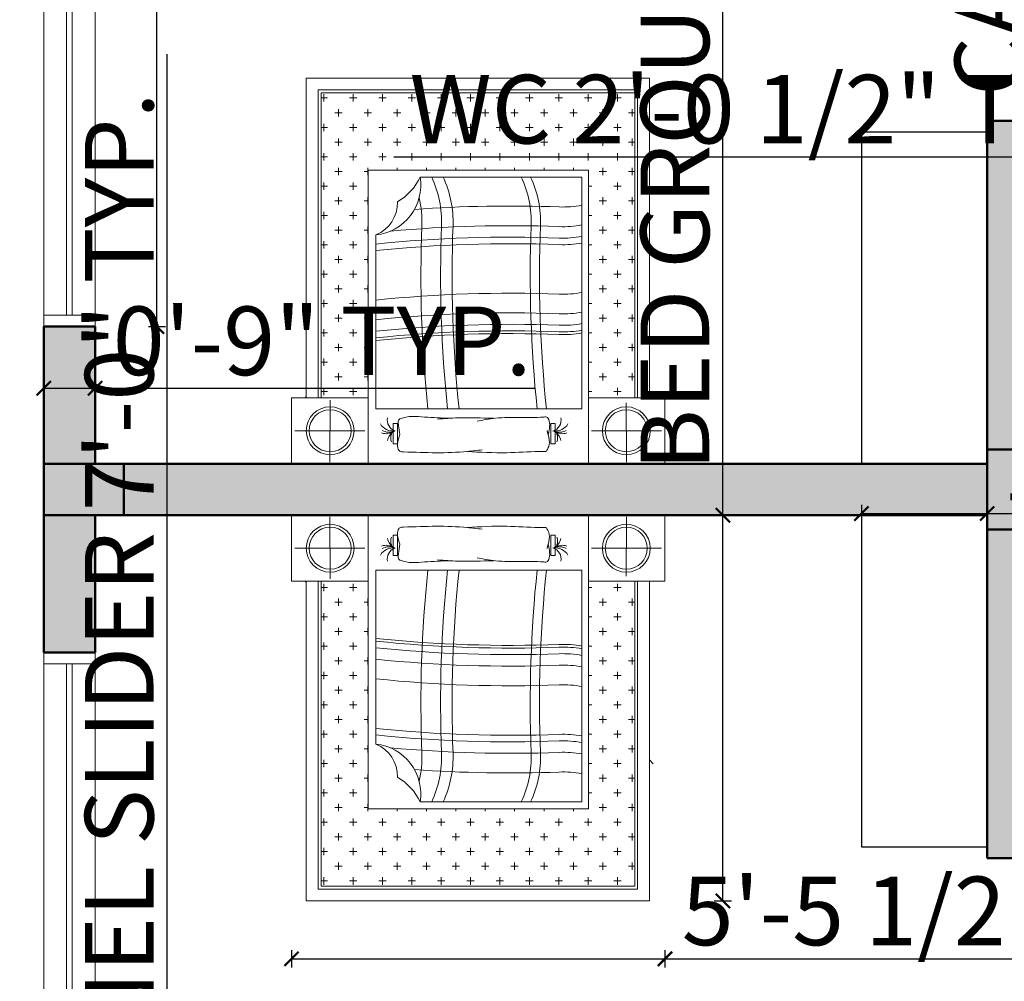
# Model space of a CAD drawing. Units: inches. Extents: x 375 to 1122, y 27 to 1069.
# Tile 71 of 155: x 494 to 667, y 499 to 667. Entities that reach past the tile are written whole.
import ezdxf

# ---------------------------------------------------------------- set-up
doc = ezdxf.new("R2010")
doc.units = ezdxf.units.IN
for name, color, linetype, lineweight in [('A-ANNO-DIMS', 2, 'Continuous', 18), ('A-COLS-PATT', 10, 'Continuous', 13), ('A-FLOR-MILL', 55, 'Continuous', 25), ('A-WALL-PATT', 252, 'Continuous', 13), ('Columns', 10, 'Continuous', 50), ('Doors', 150, 'Continuous', 25), ('Furniture', 30, 'Continuous', 18), ('Walls', 250, 'Continuous', 50), ('Windows', 122, 'Continuous', 18)]:
    doc.layers.add(name, color=color, linetype=linetype, lineweight=lineweight)
doc.styles.get("Standard").update_dxf_attribs({"font": 'arial.ttf'})
doc.dimstyles.new('ISO-25', dxfattribs={"dimtxt": 12, "dimasz": 2.5, "dimexe": 1.5, "dimexo": 1.5, "dimtad": 1, "dimdec": 1, "dimlunit": 3, "dimtxsty": 'Standard', "dimblk": 'ARCHTICK', "dimcen": 2.5, "dimadec": 0, "dimazin": 0, "dimtfac": 1, "dimtdec": 1, "dimtmove": 0, "dimatfit": 3, "dimfxl": 1.5, "dimfxlon": 1, "dimarcsym": 0})

# ---------------------------------------------------------------- blocks, each defined once
blk = doc.blocks.new('*U12')
for p, q in [((0, 0), (0, -4)), ((24, 0), (24, -4))]:
    blk.add_line(p, q)
blk.add_lwpolyline([(0, 0), (0, 24), (1.75, 24), (1.75, 0)], close=True)
blk.add_arc((0, 0), 24, 0, 90)
blk = doc.blocks.new('*U11')
for p, q in [((-24, 0), (-24, -4)), ((0, 0), (0, -4))]:
    blk.add_line(p, q)
blk.add_lwpolyline([(0, 0), (0, 24), (-1.75, 24), (-1.75, 0)], close=True)
blk.add_arc((0, 0), 24, 90, 180)
blk = doc.blocks.new('A$C52B64FF5')
for p, q in [((0.5216, 2.6276), (0, 2.6276)), ((0, 2.6276), (0, 2.1776)), ((0.2616, 2.4026), (0.2616, 2.6161)), ((0.5216, 2.1776), (0.5216, 2.6276)), ((2.0216, 2.6276), (0.5216, 2.6276)), ((0.5216, 2.6276), (0.5216, 0.6276)), ((2.5432, 2.6276), (2.0216, 2.6276)), ((2.0216, 0.6276), (2.0216, 2.6276)), ((2.0216, 2.6276), (2.0216, 2.1776)), ((2.2816, 2.4026), (2.2816, 2.6161)), ((2.5432, 2.1776), (2.5432, 2.6276)), ((0.721, 2.4927), (0.6917, 2.4927)), ((0.6917, 2.4927), (0.6917, 2.3531)), ((0.721, 2.3531), (0.721, 2.4927)), ((1.767, 2.3531), (1.767, 2.4927)), ((1.767, 2.4927), (1.7964, 2.4927)), ((1.7964, 2.4927), (1.7964, 2.3531)), ((0.2632, 2.4026), (0.0233, 2.4026)), ((0.0233, 2.4026), (0.4999, 2.4026)), ((0.2632, 2.1952), (0.2632, 2.4026)), ((0.6917, 2.3531), (0.721, 2.3531)), ((1.7964, 2.3531), (1.767, 2.3531)), ((2.5199, 2.4026), (2.0434, 2.4026)), ((2.2801, 2.2128), (2.2801, 2.4026)), ((2.2801, 2.4026), (2.5199, 2.4026)), ((0.5751, 1.0685), (0.5751, 2.2541)), ((0.5751, 2.2541), (1.9782, 2.2541)), ((1.9782, 2.2541), (1.9782, 0.6749)), ((0, 2.1776), (0.5216, 2.1776)), ((0.093, 2.1776), (0.1008, 2.1698)), ((0.1008, 0), (0.1008, 2.1776)), ((0.1808, 0.08), (0.1808, 2.1776)), ((0.2008, 0.1), (0.2008, 2.1776)), ((0.2197, 2.111), (0.2197, 2.161)), ((0.4197, 2.111), (0.4197, 2.161)), ((2.5432, 2.1776), (2.0216, 2.1776)), ((2.0216, 2.1776), (2.5432, 2.1776)), ((2.2197, 2.111), (2.2197, 2.161)), ((2.3374, 2.1776), (2.3374, 0.1)), ((2.3574, 2.1776), (2.3574, 0.08)), ((2.4374, 2.1776), (2.4374, 0)), ((0.2008, 2.136), (0.2447, 2.136)), ((0.3947, 2.136), (0.4447, 2.136)), ((2.0216, 2.136), (2.0447, 2.136)), ((2.1947, 2.136), (2.2447, 2.136)), ((0.2947, 2.036), (0.3447, 2.036)), ((0.3197, 2.011), (0.3197, 2.061)), ((0.4947, 2.036), (0.5216, 2.036)), ((0.5197, 2.011), (0.5197, 2.061)), ((2.0947, 2.036), (2.1447, 2.036)), ((2.1197, 2.011), (2.1197, 2.061)), ((2.2947, 2.036), (2.3374, 2.036)), ((2.3197, 2.011), (2.3197, 2.061)), ((0.2197, 1.911), (0.2197, 1.961)), ((0.4197, 1.911), (0.4197, 1.961)), ((2.2197, 1.911), (2.2197, 1.961)), ((0.2008, 1.936), (0.2447, 1.936)), ((0.3947, 1.936), (0.4447, 1.936)), ((2.0216, 1.936), (2.0447, 1.936)), ((2.1947, 1.936), (2.2447, 1.936)), ((0.2947, 1.836), (0.3447, 1.836)), ((0.3197, 1.811), (0.3197, 1.861)), ((0.4947, 1.836), (0.5216, 1.836)), ((0.5197, 1.811), (0.5197, 1.861)), ((2.0947, 1.836), (2.1447, 1.836)), ((2.1197, 1.811), (2.1197, 1.861)), ((2.2947, 1.836), (2.3374, 1.836)), ((2.3197, 1.811), (2.3197, 1.861)), ((0.2197, 1.711), (0.2197, 1.761)), ((0.4197, 1.711), (0.4197, 1.761)), ((2.2197, 1.711), (2.2197, 1.761)), ((0.2008, 1.736), (0.2447, 1.736)), ((0.3947, 1.736), (0.4447, 1.736)), ((2.0216, 1.736), (2.0447, 1.736)), ((2.1947, 1.736), (2.2447, 1.736)), ((0.2947, 1.636), (0.3447, 1.636)), ((0.3197, 1.611), (0.3197, 1.661)), ((0.4947, 1.636), (0.5216, 1.636)), ((0.5197, 1.611), (0.5197, 1.661)), ((2.0947, 1.636), (2.1447, 1.636)), ((2.1197, 1.611), (2.1197, 1.661)), ((2.2947, 1.636), (2.3374, 1.636)), ((2.3197, 1.611), (2.3197, 1.661)), ((0.2197, 1.511), (0.2197, 1.561)), ((0.4197, 1.511), (0.4197, 1.561)), ((2.2197, 1.511), (2.2197, 1.561)), ((0.2008, 1.536), (0.2447, 1.536)), ((0.3947, 1.536), (0.4447, 1.536)), ((2.0216, 1.536), (2.0447, 1.536)), ((2.1947, 1.536), (2.2447, 1.536)), ((0.2947, 1.436), (0.3447, 1.436)), ((0.3197, 1.411), (0.3197, 1.461)), ((0.4947, 1.436), (0.5216, 1.436)), ((0.5197, 1.411), (0.5197, 1.461)), ((2.0947, 1.436), (2.1447, 1.436)), ((2.1197, 1.411), (2.1197, 1.461)), ((2.2947, 1.436), (2.3374, 1.436)), ((2.3197, 1.411), (2.3197, 1.461)), ((0.2197, 1.311), (0.2197, 1.361)), ((0.4197, 1.311), (0.4197, 1.361)), ((2.2197, 1.311), (2.2197, 1.361)), ((0.2008, 1.336), (0.2447, 1.336)), ((0.3947, 1.336), (0.4447, 1.336)), ((2.0216, 1.336), (2.0447, 1.336)), ((2.1947, 1.336), (2.2447, 1.336)), ((0.2947, 1.236), (0.3447, 1.236)), ((0.3197, 1.211), (0.3197, 1.261)), ((0.4947, 1.236), (0.5216, 1.236)), ((0.5197, 1.211), (0.5197, 1.261)), ((2.0947, 1.236), (2.1447, 1.236)), ((2.1197, 1.211), (2.1197, 1.261)), ((2.2947, 1.236), (2.3374, 1.236)), ((2.3197, 1.211), (2.3197, 1.261)), ((0.2197, 1.111), (0.2197, 1.161)), ((0.4197, 1.111), (0.4197, 1.161)), ((2.2197, 1.111), (2.2197, 1.161)), ((0.2008, 1.136), (0.2447, 1.136)), ((0.3947, 1.136), (0.4447, 1.136)), ((2.0216, 1.136), (2.0447, 1.136)), ((2.1947, 1.136), (2.2447, 1.136)), ((0.2947, 1.036), (0.3447, 1.036)), ((0.3197, 1.011), (0.3197, 1.061)), ((0.4947, 1.036), (0.5216, 1.036)), ((0.5197, 1.011), (0.5197, 1.061)), ((2.0947, 1.036), (2.1447, 1.036)), ((2.1197, 1.011), (2.1197, 1.061)), ((2.2947, 1.036), (2.3374, 1.036)), ((2.3197, 1.011), (2.3197, 1.061)), ((0.2197, 0.911), (0.2197, 0.961)), ((0.4197, 0.911), (0.4197, 0.961)), ((2.2197, 0.911), (2.2197, 0.961)), ((2.4374, 0.9617), (2.4642, 0.935)), ((0.2008, 0.936), (0.2447, 0.936)), ((0.3947, 0.936), (0.4447, 0.936)), ((2.0216, 0.936), (2.0447, 0.936)), ((2.1947, 0.936), (2.2447, 0.936)), ((0.2947, 0.836), (0.3447, 0.836)), ((0.3197, 0.811), (0.3197, 0.861)), ((0.4947, 0.836), (0.5216, 0.836)), ((0.5197, 0.811), (0.5197, 0.861)), ((2.0947, 0.836), (2.1447, 0.836)), ((2.1197, 0.811), (2.1197, 0.861)), ((2.2947, 0.836), (2.3374, 0.836)), ((2.3197, 0.811), (2.3197, 0.861)), ((0.2197, 0.711), (0.2197, 0.761)), ((0.4197, 0.711), (0.4197, 0.761)), ((2.2197, 0.711), (2.2197, 0.761)), ((0.2008, 0.736), (0.2447, 0.736)), ((0.3947, 0.736), (0.4447, 0.736)), ((1.9782, 0.6749), (0.8764, 0.6749)), ((2.0216, 0.736), (2.0447, 0.736)), ((2.1947, 0.736), (2.2447, 0.736)), ((0.2947, 0.636), (0.3447, 0.636)), ((0.3197, 0.611), (0.3197, 0.661)), ((0.4947, 0.636), (0.5216, 0.636)), ((0.5197, 0.611), (0.5197, 0.661)), ((0.5216, 0.6276), (2.0216, 0.6276)), ((0.7197, 0.611), (0.7197, 0.6276)), ((0.9197, 0.611), (0.9197, 0.6276)), ((1.1197, 0.611), (1.1197, 0.6276)), ((1.3197, 0.611), (1.3197, 0.6276)), ((1.5197, 0.611), (1.5197, 0.6276)), ((1.7197, 0.611), (1.7197, 0.6276)), ((1.9197, 0.611), (1.9197, 0.6276)), ((2.0947, 0.636), (2.1447, 0.636)), ((2.1197, 0.611), (2.1197, 0.661)), ((2.2947, 0.636), (2.3374, 0.636)), ((2.3197, 0.611), (2.3197, 0.661)), ((0.2197, 0.511), (0.2197, 0.561)), ((0.4197, 0.511), (0.4197, 0.561)), ((0.6197, 0.511), (0.6197, 0.561)), ((0.8197, 0.511), (0.8197, 0.561)), ((1.0197, 0.511), (1.0197, 0.561)), ((1.2197, 0.511), (1.2197, 0.561)), ((1.4197, 0.511), (1.4197, 0.561)), ((1.6197, 0.511), (1.6197, 0.561)), ((1.8197, 0.511), (1.8197, 0.561)), ((2.0197, 0.511), (2.0197, 0.561)), ((2.2197, 0.511), (2.2197, 0.561)), ((0.2008, 0.536), (0.2447, 0.536)), ((0.3947, 0.536), (0.4447, 0.536)), ((0.5947, 0.536), (0.6447, 0.536)), ((0.7947, 0.536), (0.8447, 0.536)), ((0.9947, 0.536), (1.0447, 0.536)), ((1.1947, 0.536), (1.2447, 0.536)), ((1.3947, 0.536), (1.4447, 0.536)), ((1.5947, 0.536), (1.6447, 0.536)), ((1.7947, 0.536), (1.8447, 0.536)), ((1.9947, 0.536), (2.0447, 0.536)), ((2.1947, 0.536), (2.2447, 0.536)), ((0.2947, 0.436), (0.3447, 0.436)), ((0.3197, 0.411), (0.3197, 0.461)), ((0.4947, 0.436), (0.5447, 0.436)), ((0.5197, 0.411), (0.5197, 0.461)), ((0.6947, 0.436), (0.7447, 0.436)), ((0.7197, 0.411), (0.7197, 0.461)), ((0.8947, 0.436), (0.9447, 0.436)), ((0.9197, 0.411), (0.9197, 0.461)), ((1.0947, 0.436), (1.1447, 0.436)), ((1.1197, 0.411), (1.1197, 0.461)), ((1.2947, 0.436), (1.3447, 0.436)), ((1.3197, 0.411), (1.3197, 0.461)), ((1.4947, 0.436), (1.5447, 0.436)), ((1.5197, 0.411), (1.5197, 0.461)), ((1.6947, 0.436), (1.7447, 0.436)), ((1.7197, 0.411), (1.7197, 0.461)), ((1.8947, 0.436), (1.9447, 0.436)), ((1.9197, 0.411), (1.9197, 0.461)), ((2.0947, 0.436), (2.1447, 0.436)), ((2.1197, 0.411), (2.1197, 0.461)), ((2.2947, 0.436), (2.3374, 0.436)), ((2.3197, 0.411), (2.3197, 0.461)), ((0.2008, 0.336), (0.2447, 0.336)), ((0.2197, 0.311), (0.2197, 0.361)), ((0.3947, 0.336), (0.4447, 0.336)), ((0.4197, 0.311), (0.4197, 0.361)), ((0.5947, 0.336), (0.6447, 0.336)), ((0.6197, 0.311), (0.6197, 0.361)), ((0.7947, 0.336), (0.8447, 0.336)), ((0.8197, 0.311), (0.8197, 0.361)), ((0.9947, 0.336), (1.0447, 0.336)), ((1.0197, 0.311), (1.0197, 0.361)), ((1.1947, 0.336), (1.2447, 0.336)), ((1.2197, 0.311), (1.2197, 0.361)), ((1.3947, 0.336), (1.4447, 0.336)), ((1.4197, 0.311), (1.4197, 0.361)), ((1.5947, 0.336), (1.6447, 0.336)), ((1.6197, 0.311), (1.6197, 0.361)), ((1.7947, 0.336), (1.8447, 0.336)), ((1.8197, 0.311), (1.8197, 0.361)), ((1.9947, 0.336), (2.0447, 0.336)), ((2.0197, 0.311), (2.0197, 0.361)), ((2.1947, 0.336), (2.2447, 0.336)), ((2.2197, 0.311), (2.2197, 0.361)), ((0.2947, 0.236), (0.3447, 0.236)), ((0.3197, 0.211), (0.3197, 0.261)), ((0.4947, 0.236), (0.5447, 0.236)), ((0.5197, 0.211), (0.5197, 0.261)), ((0.6947, 0.236), (0.7447, 0.236)), ((0.7197, 0.211), (0.7197, 0.261)), ((0.8947, 0.236), (0.9447, 0.236)), ((0.9197, 0.211), (0.9197, 0.261)), ((1.0947, 0.236), (1.1447, 0.236)), ((1.1197, 0.211), (1.1197, 0.261)), ((1.2947, 0.236), (1.3447, 0.236)), ((1.3197, 0.211), (1.3197, 0.261)), ((1.4947, 0.236), (1.5447, 0.236)), ((1.5197, 0.211), (1.5197, 0.261)), ((1.6947, 0.236), (1.7447, 0.236)), ((1.7197, 0.211), (1.7197, 0.261)), ((1.8947, 0.236), (1.9447, 0.236)), ((1.9197, 0.211), (1.9197, 0.261)), ((2.0947, 0.236), (2.1447, 0.236)), ((2.1197, 0.211), (2.1197, 0.261)), ((2.2947, 0.236), (2.3374, 0.236)), ((2.3197, 0.211), (2.3197, 0.261)), ((0.2008, 0.136), (0.2447, 0.136)), ((0.2197, 0.111), (0.2197, 0.161)), ((0.3947, 0.136), (0.4447, 0.136)), ((0.4197, 0.111), (0.4197, 0.161)), ((0.5947, 0.136), (0.6447, 0.136)), ((0.6197, 0.111), (0.6197, 0.161)), ((0.7947, 0.136), (0.8447, 0.136)), ((0.8197, 0.111), (0.8197, 0.161)), ((0.9947, 0.136), (1.0447, 0.136)), ((1.0197, 0.111), (1.0197, 0.161)), ((1.1947, 0.136), (1.2447, 0.136)), ((1.2197, 0.111), (1.2197, 0.161)), ((1.3947, 0.136), (1.4447, 0.136)), ((1.4197, 0.111), (1.4197, 0.161)), ((1.5947, 0.136), (1.6447, 0.136)), ((1.6197, 0.111), (1.6197, 0.161)), ((1.7947, 0.136), (1.8447, 0.136)), ((1.8197, 0.111), (1.8197, 0.161)), ((1.9947, 0.136), (2.0447, 0.136)), ((2.0197, 0.111), (2.0197, 0.161)), ((2.1947, 0.136), (2.2447, 0.136)), ((2.2197, 0.111), (2.2197, 0.161)), ((2.3574, 0.08), (0.1808, 0.08)), ((2.3374, 0.1), (0.2008, 0.1)), ((2.4374, 0), (0.1008, 0))]:
    blk.add_line(p, q)
for centre, radius in [((0.2632, 2.4026), 0.1631), ((2.2801, 2.4026), 0.1631), ((0.2632, 2.4026), 0.1431), ((2.2801, 2.4026), 0.1431)]:
    blk.add_circle(centre, radius)
for centre, radius, start, end in [((0.6442, 2.3154), 0.1072, 59.2174, 107.24009), ((0.7523, 2.4916), 0.1013, 192.77399, 239.2386), ((0.7566, 2.4523), 0.0808, 161.45592, 221.5545), ((1.7358, 2.4916), 0.1013, 300.7614, 347.22601), ((1.8439, 2.3154), 0.1072, 72.75991, 120.7826), ((1.7315, 2.4523), 0.0808, 318.4455, 18.54408), ((0.6895, 2.3063), 0.098, 80.94857, 149.48786), ((0.6646, 2.3215), 0.0913, 67.83977, 120.48585), ((0.7294, 2.33), 0.0776, 109.26419, 192.26691), ((1.7587, 2.33), 0.0776, 347.73309, 73.88358), ((1.7986, 2.3063), 0.098, 30.51214, 99.05143), ((1.8235, 2.3215), 0.0913, 59.51415, 112.16023), ((9.7293, 1.3409), 8.8479, 174.07538, 182.16616), ((9.8633, 1.3409), 8.8479, 174.07538, 182.16616), ((9.9414, 1.3409), 8.8479, 174.07538, 182.16616), ((10.4736, 1.3409), 8.8479, 174.07538, 182.16616), ((10.5369, 1.3409), 8.8479, 174.07538, 182.16616), ((1.4884, 10.5889), 8.8479, 264.07538, 272.16616), ((1.4884, 10.5702), 8.8479, 264.07538, 272.16616), ((1.85, 1.0282), 0.7196, 79.7409, 92.16616), ((1.4884, 10.5256), 8.8479, 264.07538, 272.16616), ((1.85, 1.0096), 0.7196, 79.7409, 92.16616), ((1.85, 0.965), 0.7196, 79.7409, 92.16616), ((1.4884, 10.4474), 8.8479, 264.07538, 272.16616), ((1.85, 0.8868), 0.7196, 79.7409, 92.16616), ((1.4884, 10.3135), 8.8479, 264.07538, 272.16616), ((1.85, 0.7528), 0.7196, 79.7409, 92.16616), ((1.4884, 9.9764), 8.8479, 264.07538, 272.16616), ((1.4884, 9.9317), 8.8479, 264.07538, 272.16616), ((1.85, 0.4158), 0.7196, 79.7409, 92.16616), ((1.85, 0.3711), 0.7196, 79.7409, 92.16616), ((0.4865, 0.8516), 0.2343, 358.03681, 67.7864), ((0.5391, 0.7288), 0.3416, 350.92672, 83.95649), ((1.4884, 9.8536), 8.8479, 264.70583, 272.16616), ((0.1687, 0.9792), 0.7196, 346.86533, 2.16616), ((0.3027, 0.9792), 0.7196, 334.98359, 2.16616), ((0.3808, 0.9792), 0.7196, 334.98359, 2.16616), ((0.913, 0.9792), 0.7196, 334.98359, 2.16616), ((0.9763, 0.9792), 0.7196, 334.98359, 2.16616), ((1.85, 0.293), 0.7196, 79.7409, 92.16616), ((1.4884, 9.7196), 8.8479, 265.77852, 272.16616), ((1.85, 0.159), 0.7196, 79.7409, 92.16616), ((0.5285, 0.5098), 0.3852, 25.3912, 60.06861)]:
    blk.add_arc(centre, radius, start, end)
for points, knots in [([(0.7373, 2.4293), (0.7344, 2.4386), (0.7239, 2.472), (0.715, 2.518), (0.7414, 2.5459), (0.9088, 2.5514), (1.0864, 2.5586), (1.2642, 2.5365), (1.2976, 2.5323)], [0, 0, 0, 0, 0.0298664, 0.1071619, 0.1152509, 0.1416099, 0.5761797, 0.6768951, 0.6768951, 0.6768951, 0.6768951]), ([(1.1947, 2.5438), (1.2853, 2.549), (1.4483, 2.5585), (1.6283, 2.5432), (1.7179, 2.5437), (1.7351, 2.5438)], [0, 0, 0, 0, 0.2717358, 0.4891854, 0.5406465, 0.5406465, 0.5406465, 0.5406465]), ([(1.7351, 2.5438), (1.7416, 2.5321), (1.759, 2.5014), (1.7583, 2.4623), (1.7348, 2.3817), (1.7455, 2.4145), (1.7494, 2.4265)], [0, 0, 0, 0, 0.0383771, 0.1013156, 0.1484959, 0.1756343, 0.1756343, 0.1756343, 0.1756343]), ([(1.0802, 2.3175), (1.0225, 2.3155), (0.9099, 2.3116), (0.7905, 2.2985), (0.7234, 2.3279), (0.7309, 2.3766), (0.7348, 2.4091), (0.7373, 2.4293)], [0, 0, 0, 0, 0.1744349, 0.3406483, 0.347042, 0.3874998, 0.4538558, 0.4538558, 0.4538558, 0.4538558]), ([(1.7494, 2.4265), (1.7531, 2.4084), (1.7601, 2.3751), (1.7573, 2.3363), (1.7437, 2.3065), (1.6676, 2.315), (1.559, 2.3108), (1.4028, 2.3119), (1.305, 2.3301), (1.2633, 2.3378)], [0, 0, 0, 0, 0.0550284, 0.1011576, 0.1178362, 0.1437253, 0.3009935, 0.4726259, 0.6000038, 0.6000038, 0.6000038, 0.6000038]), ([(1.3748, 2.3178), (1.2947, 2.315), (1.1678, 2.3105), (1.0413, 2.32), (0.9946, 2.3235)], [0, 0, 0, 0, 0.2401688, 0.38052, 0.38052, 0.38052, 0.38052])]:
    blk.add_open_spline(points, degree=3, knots=knots)
blk = doc.blocks.new('WINDOW-72IN')
for p, q in [((4, 70), (4, 2)), ((5, 70), (5, 2))]:
    blk.add_line(p, q)
blk.add_lwpolyline([(9, 0), (0, 0), (0, 72), (9, 72)], close=True)
for points in [[(0, 70), (9, 70)], [(9, 2), (0, 2)]]:
    blk.add_lwpolyline(points)
blk = doc.blocks.new('COLUMN-14X9IN')
blk.add_lwpolyline([(0, 0), (14, 0), (14, 9), (0, 9)], close=True)
blk = doc.blocks.new('BEDROOM-CABINET-22X58IN')
blk.add_lwpolyline([(0, 0), (22, 0), (22, 58), (0, 58)], close=True)
blk = doc.blocks.new('_ArchTick')
at = {"color": 0, "linetype": 'ByBlock', "const_width": 0.15}
blk.add_lwpolyline([(-0.5, -0.5), (0.5, 0.5)], dxfattribs=at)
blk = doc.blocks.new('*D43')
at = {"layer": 'A-ANNO-DIMS', "color": 0, "lineweight": -2, "transparency": 16777216}
for p, q in [((617.28, 580.53), (617.28, 790.11)), ((615.78, 580.53), (618.78, 580.53)), ((617.28, 513.06), (617.28, 580.53)), ((615.78, 513.06), (618.78, 513.06))]:
    blk.add_line(p, q, dxfattribs=at)
at = {"layer": 'Defpoints', "color": 0, "transparency": 16777216}
for p in [(607.16, 580.53), (617.28, 580.53), (607.16, 513.06)]:
    blk.add_point(p, dxfattribs=at)
at = {"layer": 'A-ANNO-DIMS', "color": 0, "lineweight": -2, "transparency": 16777216, "xscale": 2.5, "yscale": 2.5, "zscale": 2.5}
for p, rotation in [((617.28, 580.53), 90), ((617.28, 513.06), 270)]:
    blk.add_blockref('_ArchTick', p, dxfattribs=dict(at, rotation=rotation))
at = {"layer": 'A-ANNO-DIMS', "color": 0, "transparency": 16777216, "insert": (610.45, 686.57), "char_height": 12, "attachment_point": 5, "rotation": 90}
blk.add_mtext('BED GROUP 5\'-7 1/2" TYP.', dxfattribs=at)
blk = doc.blocks.new('*D44')
at = {"layer": 'A-ANNO-DIMS', "color": 0, "lineweight": -2, "transparency": 16777216}
for p, q in [((541.85, 504.43), (541.85, 501.43)), ((541.85, 502.93), (607.16, 502.93)), ((607.16, 504.43), (607.16, 501.43)), ((607.16, 502.93), (712.02, 502.93))]:
    blk.add_line(p, q, dxfattribs=at)
at = {"layer": 'Defpoints', "color": 0, "transparency": 16777216}
for p in [(541.85, 513.06), (607.16, 513.06), (607.16, 502.93)]:
    blk.add_point(p, dxfattribs=at)
at = {"layer": 'A-ANNO-DIMS', "color": 0, "lineweight": -2, "transparency": 16777216, "xscale": 2.5, "yscale": 2.5, "zscale": 2.5, "rotation": 180}
blk.add_blockref('_ArchTick', (541.85, 502.93), dxfattribs=at)
at = {"layer": 'A-ANNO-DIMS', "color": 0, "lineweight": -2, "transparency": 16777216, "xscale": 2.5, "yscale": 2.5, "zscale": 2.5}
blk.add_blockref('_ArchTick', (607.16, 502.93), dxfattribs=at)
at = {"layer": 'A-ANNO-DIMS', "color": 0, "transparency": 16777216, "insert": (660.84, 509.76), "char_height": 12, "attachment_point": 5}
blk.add_mtext('5\'-5 1/2" TYP.', dxfattribs=at)
blk = doc.blocks.new('*D45')
at = {"layer": 'A-ANNO-DIMS', "color": 0, "lineweight": -2, "transparency": 16777216}
for p, q in [((697.69, 641.67), (697.69, 644.67)), ((722.01, 641.67), (722.01, 644.67)), ((697.69, 643.17), (559.76, 643.17)), ((722.01, 643.17), (697.69, 643.17))]:
    blk.add_line(p, q, dxfattribs=at)
at = {"layer": 'Defpoints', "color": 0, "transparency": 16777216}
for p in [(697.69, 643.17), (697.69, 639.53), (722.01, 639.53)]:
    blk.add_point(p, dxfattribs=at)
at = {"layer": 'A-ANNO-DIMS', "color": 0, "lineweight": -2, "transparency": 16777216, "xscale": 2.5, "yscale": 2.5, "zscale": 2.5, "rotation": 180}
blk.add_blockref('_ArchTick', (697.69, 643.17), dxfattribs=at)
at = {"layer": 'A-ANNO-DIMS', "color": 0, "lineweight": -2, "transparency": 16777216, "xscale": 2.5, "yscale": 2.5, "zscale": 2.5}
blk.add_blockref('_ArchTick', (722.01, 643.17), dxfattribs=at)
at = {"layer": 'A-ANNO-DIMS', "color": 0, "transparency": 16777216, "insert": (627.47, 650), "char_height": 12, "attachment_point": 5}
blk.add_mtext('WC 2\'-0 1/2" TYP.', dxfattribs=at)
blk = doc.blocks.new('*D69')
at = {"layer": 'A-ANNO-DIMS', "color": 0, "lineweight": -2, "transparency": 16777216}
for p, q in [((518.31, 685.53), (518.31, 841.13)), ((516.81, 685.53), (519.81, 685.53)), ((518.31, 613.53), (518.31, 685.53)), ((516.81, 613.53), (519.81, 613.53))]:
    blk.add_line(p, q, dxfattribs=at)
at = {"layer": 'Defpoints', "color": 0, "transparency": 16777216}
for p in [(507.51, 685.53), (518.31, 685.53), (507.51, 613.53)]:
    blk.add_point(p, dxfattribs=at)
at = {"layer": 'A-ANNO-DIMS', "color": 0, "lineweight": -2, "transparency": 16777216, "xscale": 2.5, "yscale": 2.5, "zscale": 2.5}
for p, rotation in [((518.31, 685.53), 90), ((518.31, 613.53), 270)]:
    blk.add_blockref('_ArchTick', p, dxfattribs=dict(at, rotation=rotation))
at = {"layer": 'A-ANNO-DIMS', "color": 0, "transparency": 16777216, "insert": (511.47, 764.58), "char_height": 12, "attachment_point": 5, "rotation": 90}
blk.add_mtext('WINDOW 6\'-0" TYP.', dxfattribs=at)
blk = doc.blocks.new('*D70')
at = {"layer": 'A-ANNO-DIMS', "color": 0, "lineweight": -2, "transparency": 16777216}
for p, q in [((498.51, 604.23), (498.51, 601.23)), ((498.51, 602.73), (507.51, 602.73)), ((507.51, 604.23), (507.51, 601.23)), ((507.51, 602.73), (584.4, 602.73))]:
    blk.add_line(p, q, dxfattribs=at)
at = {"layer": 'Defpoints', "color": 0, "transparency": 16777216}
for p in [(498.51, 613.53), (507.51, 613.53), (507.51, 602.73)]:
    blk.add_point(p, dxfattribs=at)
at = {"layer": 'A-ANNO-DIMS', "color": 0, "lineweight": -2, "transparency": 16777216, "xscale": 2.5, "yscale": 2.5, "zscale": 2.5, "rotation": 180}
blk.add_blockref('_ArchTick', (498.51, 602.73), dxfattribs=at)
at = {"layer": 'A-ANNO-DIMS', "color": 0, "lineweight": -2, "transparency": 16777216, "xscale": 2.5, "yscale": 2.5, "zscale": 2.5}
blk.add_blockref('_ArchTick', (507.51, 602.73), dxfattribs=at)
at = {"layer": 'A-ANNO-DIMS', "color": 0, "transparency": 16777216, "insert": (547.21, 609.48), "char_height": 12, "attachment_point": 5}
blk.add_mtext('0\'-9" TYP.', dxfattribs=at)
blk = doc.blocks.new('*D71')
at = {"layer": 'A-ANNO-DIMS', "color": 0, "lineweight": -2, "transparency": 16777216}
for p, q in [((520.11, 444.53), (520.11, 661.17)), ((518.61, 444.53), (521.61, 444.53)), ((520.11, 360.53), (520.11, 444.53)), ((518.61, 360.53), (521.61, 360.53))]:
    blk.add_line(p, q, dxfattribs=at)
at = {"layer": 'Defpoints', "color": 0, "transparency": 16777216}
for p in [(507.51, 444.53), (520.11, 444.53), (507.51, 360.53)]:
    blk.add_point(p, dxfattribs=at)
at = {"layer": 'A-ANNO-DIMS', "color": 0, "lineweight": -2, "transparency": 16777216, "xscale": 2.5, "yscale": 2.5, "zscale": 2.5}
for p, rotation in [((520.11, 444.53), 90), ((520.11, 360.53), 270)]:
    blk.add_blockref('_ArchTick', p, dxfattribs=dict(at, rotation=rotation))
at = {"layer": 'A-ANNO-DIMS', "color": 0, "transparency": 16777216, "insert": (513.27, 554.1), "char_height": 12, "attachment_point": 5, "rotation": 90}
blk.add_mtext('3-PANEL SLIDER 7\'-0" TYP.', dxfattribs=at)
blk = doc.blocks.new('*D79')
at = {"layer": 'A-ANNO-DIMS', "color": 0, "lineweight": -2, "transparency": 16777216}
for p, q in [((672.21, 647.53), (672.21, 810.92)), ((670.71, 647.53), (673.71, 647.53)), ((672.21, 589.53), (672.21, 647.53)), ((670.71, 589.53), (673.71, 589.53))]:
    blk.add_line(p, q, dxfattribs=at)
at = {"layer": 'Defpoints', "color": 0, "transparency": 16777216}
for p in [(663.51, 647.53), (672.21, 647.53), (663.51, 589.53)]:
    blk.add_point(p, dxfattribs=at)
at = {"layer": 'A-ANNO-DIMS', "color": 0, "lineweight": -2, "transparency": 16777216, "xscale": 2.5, "yscale": 2.5, "zscale": 2.5}
for p, rotation in [((672.21, 647.53), 90), ((672.21, 589.53), 270)]:
    blk.add_blockref('_ArchTick', p, dxfattribs=dict(at, rotation=rotation))
at = {"layer": 'A-ANNO-DIMS', "color": 0, "transparency": 16777216, "insert": (665.38, 730.47), "char_height": 12, "attachment_point": 5, "rotation": 90}
blk.add_mtext('CABINET 4\'-10" TYP.', dxfattribs=at)
blk = doc.blocks.new('*D80')
at = {"layer": 'A-ANNO-DIMS', "color": 0, "lineweight": -2, "transparency": 16777216}
for p, q in [((641.51, 582.33), (641.51, 579.33)), ((663.51, 582.33), (663.51, 579.33)), ((641.51, 580.83), (663.51, 580.83)), ((663.51, 580.83), (748.6, 580.83))]:
    blk.add_line(p, q, dxfattribs=at)
at = {"layer": 'Defpoints', "color": 0, "transparency": 16777216}
for p in [(641.51, 589.53), (663.51, 589.53), (663.51, 580.83)]:
    blk.add_point(p, dxfattribs=at)
at = {"layer": 'A-ANNO-DIMS', "color": 0, "lineweight": -2, "transparency": 16777216, "xscale": 2.5, "yscale": 2.5, "zscale": 2.5, "rotation": 180}
blk.add_blockref('_ArchTick', (641.51, 580.83), dxfattribs=at)
at = {"layer": 'A-ANNO-DIMS', "color": 0, "lineweight": -2, "transparency": 16777216, "xscale": 2.5, "yscale": 2.5, "zscale": 2.5}
blk.add_blockref('_ArchTick', (663.51, 580.83), dxfattribs=at)
at = {"layer": 'A-ANNO-DIMS', "color": 0, "transparency": 16777216, "insert": (707.3, 587.58), "char_height": 12, "attachment_point": 5}
blk.add_mtext('1\'-10" TYP.', dxfattribs=at)
blk = doc.blocks.new('*D82')
at = {"layer": 'A-ANNO-DIMS', "color": 0, "lineweight": -2, "transparency": 16777216}
for p, q in [((401.51, 1009.53), (398.51, 1009.53)), ((400.01, 160.53), (400.01, 1009.53)), ((401.51, 160.53), (398.51, 160.53))]:
    blk.add_line(p, q, dxfattribs=at)
at = {"layer": 'Defpoints', "color": 0, "transparency": 16777216}
for p in [(400.01, 1009.53), (630.53, 1009.53), (630.53, 160.53)]:
    blk.add_point(p, dxfattribs=at)
at = {"layer": 'A-ANNO-DIMS', "color": 0, "lineweight": -2, "transparency": 16777216, "xscale": 2.5, "yscale": 2.5, "zscale": 2.5}
for p, rotation in [((400.01, 1009.53), 90), ((400.01, 160.53), 270)]:
    blk.add_blockref('_ArchTick', p, dxfattribs=dict(at, rotation=rotation))
at = {"layer": 'A-ANNO-DIMS', "color": 0, "transparency": 16777216, "insert": (393.26, 585.03), "char_height": 12, "attachment_point": 5, "rotation": 90}
blk.add_mtext('70\'-9"', dxfattribs=at)
blk = doc.blocks.new('*D90')
at = {"layer": 'A-ANNO-DIMS', "color": 0, "lineweight": -2, "transparency": 16777216}
for p, q in [((401.51, 574.53), (398.51, 574.53)), ((400.01, 502.53), (400.01, 574.53)), ((401.51, 502.53), (398.51, 502.53))]:
    blk.add_line(p, q, dxfattribs=at)
at = {"layer": 'Defpoints', "color": 0, "transparency": 16777216}
for p in [(400.01, 574.53), (863.01, 574.53), (863.01, 502.53)]:
    blk.add_point(p, dxfattribs=at)
at = {"layer": 'A-ANNO-DIMS', "color": 0, "lineweight": -2, "transparency": 16777216, "xscale": 2.5, "yscale": 2.5, "zscale": 2.5}
for p, rotation in [((400.01, 574.53), 90), ((400.01, 502.53), 270)]:
    blk.add_blockref('_ArchTick', p, dxfattribs=dict(at, rotation=rotation))
at = {"layer": 'A-ANNO-DIMS', "color": 0, "transparency": 16777216, "insert": (393.26, 538.53), "char_height": 12, "attachment_point": 5, "rotation": 90}
blk.add_mtext('6\'-0"', dxfattribs=at)
blk = doc.blocks.new('*D92')
at = {"layer": 'A-ANNO-DIMS', "color": 0, "lineweight": -2, "transparency": 16777216}
for p, q in [((621.51, 1052.53), (621.51, 1055.53)), ((621.51, 1054.03), (657.51, 1054.03)), ((657.51, 1052.53), (657.51, 1055.53))]:
    blk.add_line(p, q, dxfattribs=at)
at = {"layer": 'Defpoints', "color": 0, "transparency": 16777216}
for p in [(657.51, 1054.03), (621.51, 460.53), (657.51, 460.53)]:
    blk.add_point(p, dxfattribs=at)
at = {"layer": 'A-ANNO-DIMS', "color": 0, "lineweight": -2, "transparency": 16777216, "xscale": 2.5, "yscale": 2.5, "zscale": 2.5, "rotation": 180}
blk.add_blockref('_ArchTick', (621.51, 1054.03), dxfattribs=at)
at = {"layer": 'A-ANNO-DIMS', "color": 0, "lineweight": -2, "transparency": 16777216, "xscale": 2.5, "yscale": 2.5, "zscale": 2.5}
blk.add_blockref('_ArchTick', (657.51, 1054.03), dxfattribs=at)
at = {"layer": 'A-ANNO-DIMS', "color": 0, "transparency": 16777216, "insert": (639.51, 1060.78), "char_height": 12, "attachment_point": 5}
blk.add_mtext('3\'-0"', dxfattribs=at)
blk = doc.blocks.new('*D93')
at = {"layer": 'A-ANNO-DIMS', "color": 0, "lineweight": -2, "transparency": 16777216}
for p, q in [((400.01, 673.53), (400.01, 709.38)), ((401.51, 673.53), (398.51, 673.53)), ((400.01, 649.53), (400.01, 673.53)), ((401.51, 649.53), (398.51, 649.53))]:
    blk.add_line(p, q, dxfattribs=at)
at = {"layer": 'Defpoints', "color": 0, "transparency": 16777216}
for p in [(400.01, 673.53), (663.51, 673.53), (663.51, 649.53)]:
    blk.add_point(p, dxfattribs=at)
at = {"layer": 'A-ANNO-DIMS', "color": 0, "lineweight": -2, "transparency": 16777216, "xscale": 2.5, "yscale": 2.5, "zscale": 2.5}
for p, rotation in [((400.01, 673.53), 90), ((400.01, 649.53), 270)]:
    blk.add_blockref('_ArchTick', p, dxfattribs=dict(at, rotation=rotation))
at = {"layer": 'A-ANNO-DIMS', "color": 0, "transparency": 16777216, "insert": (393.26, 692.7), "char_height": 12, "attachment_point": 5, "rotation": 90}
blk.add_mtext('2\'-0"', dxfattribs=at)

msp = doc.modelspace()

# ---------------------------------------------------------------- hatches: boundary and pattern name
at = {"layer": 'A-COLS-PATT'}
h = msp.add_hatch(color=256, dxfattribs=at)
h.dxf.hatch_style = 1
h.paths.add_polyline_path([(512.51, 982.53), (498.51, 982.53), (498.51, 973.53), (512.51, 973.53)])
h.paths.add_polyline_path([(666.51, 982.53), (652.51, 982.53), (652.51, 973.53), (666.51, 973.53)])
h.paths.add_polyline_path([(802.01, 982.53), (788.01, 982.53), (788.01, 973.53), (802.01, 973.53)])
h.paths.add_polyline_path([(932.01, 982.53), (918.01, 982.53), (918.01, 973.53), (932.01, 973.53)])
h.paths.add_polyline_path([(507.51, 841.53), (498.51, 841.53), (498.51, 827.53), (507.51, 827.53)])
h.paths.add_polyline_path([(666.51, 844.53), (652.51, 844.53), (652.51, 835.53), (666.51, 835.53)])
h.paths.add_polyline_path([(802.01, 814.53), (788.01, 814.53), (788.01, 805.53), (802.01, 805.53)])
h.paths.add_polyline_path([(932.01, 814.53), (918.01, 814.53), (918.01, 805.53), (932.01, 805.53)])
h.paths.add_polyline_path([(507.51, 719.53), (498.51, 719.53), (498.51, 705.53), (507.51, 705.53)])
h.paths.add_polyline_path([(731.01, 676.53), (722.01, 676.53), (722.01, 662.53), (731.01, 662.53)])
h.paths.add_polyline_path([(802.01, 676.53), (788.01, 676.53), (788.01, 667.53), (802.01, 667.53)])
h.paths.add_polyline_path([(932.01, 676.53), (918.01, 676.53), (918.01, 667.53), (932.01, 667.53)])
h.paths.add_polyline_path([(932.01, 583.53), (918.01, 583.53), (918.01, 574.53), (932.01, 574.53)])
h.paths.add_polyline_path([(868.01, 583.53), (854.01, 583.53), (854.01, 574.53), (868.01, 574.53)])
h.paths.add_polyline_path([(868.01, 502.53), (854.01, 502.53), (854.01, 493.53), (868.01, 493.53)])
h.paths.add_polyline_path([(932.01, 502.53), (918.01, 502.53), (918.01, 493.53), (932.01, 493.53)])
h.paths.add_polyline_path([(672.51, 592.03), (663.51, 592.03), (663.51, 578.03), (672.51, 578.03)])
h.paths.add_polyline_path([(512.51, 589.53), (498.51, 589.53), (498.51, 580.53), (512.51, 580.53)])
h.paths.add_polyline_path([(507.51, 464.53), (498.51, 464.53), (498.51, 450.53), (507.51, 450.53)])
h.paths.add_polyline_path([(731.01, 507.53), (722.01, 507.53), (722.01, 493.53), (731.01, 493.53)])
h.paths.add_polyline_path([(802.01, 502.53), (788.01, 502.53), (788.01, 493.53), (802.01, 493.53)])
h.paths.add_polyline_path([(507.51, 342.53), (498.51, 342.53), (498.51, 328.53), (507.51, 328.53)])
h.paths.add_polyline_path([(512.51, 196.53), (498.51, 196.53), (498.51, 187.53), (512.51, 187.53)])
h.paths.add_polyline_path([(666.51, 334.53), (652.51, 334.53), (652.51, 325.53), (666.51, 325.53)])
h.paths.add_polyline_path([(666.51, 196.53), (652.51, 196.53), (652.51, 187.53), (666.51, 187.53)])
h.paths.add_polyline_path([(805.01, 196.53), (791.01, 196.53), (791.01, 187.53), (805.01, 187.53)])
h.paths.add_polyline_path([(932.01, 196.53), (918.01, 196.53), (918.01, 187.53), (932.01, 187.53)])
h.paths.add_polyline_path([(932.01, 334.53), (918.01, 334.53), (918.01, 325.53), (932.01, 325.53)])
h.paths.add_polyline_path([(805.01, 334.53), (791.01, 334.53), (791.01, 325.53), (805.01, 325.53)])
at = {"layer": 'A-WALL-PATT'}
h = msp.add_hatch(color=256, dxfattribs=at)
h.dxf.hatch_style = 1
h.paths.add_polyline_path([(962.01, 388.53), (989.01, 388.53), (989.01, 394.53), (962.01, 394.53), (932.01, 394.53), (932.01, 397.53), (923.01, 397.53), (923.01, 394.53), (842.01, 394.53), (842.01, 334.53), (839.51, 334.53), (839.51, 328.53), (854.01, 328.53), (854.01, 334.53), (848.01, 334.53), (848.01, 388.53), (953.01, 388.53), (953.01, 356.08), (962.01, 356.08), (962.01, 358.55), (989.01, 358.55), (989.01, 364.55), (962.01, 364.55)])
h.paths.add_polyline_path([(989.01, 502.53), (932.01, 502.53), (932.01, 583.53), (932.01, 593.53), (923.01, 593.53), (923.01, 583.53), (854.01, 583.53), (854.01, 556.53), (863.01, 556.53), (863.01, 574.53), (923.01, 574.53), (923.01, 502.53), (863.01, 502.53), (863.01, 520.53), (854.01, 520.53), (854.01, 502.53), (773.01, 502.53), (773.01, 493.53), (788.01, 493.53), (788.01, 402.03), (722.01, 402.03), (722.01, 373.53), (728.01, 373.53), (728.01, 396.03), (788.01, 396.03), (788.01, 373.53), (794.01, 373.53), (794.01, 430.53), (814.01, 430.53), (814.01, 436.53), (794.01, 436.53), (794.01, 493.53), (923.01, 493.53), (923.01, 487.53), (932.01, 487.53), (932.01, 493.53), (983.01, 493.53), (983.01, 473.53), (989.01, 473.53)])
h.paths.add_polyline_path([(797.01, 325.53), (805.01, 325.53), (805.01, 328.53), (807.51, 328.53), (807.51, 334.53), (791.01, 334.53), (791.01, 226.53), (770.76, 226.53), (770.76, 217.53), (791.01, 217.53), (791.01, 187.53), (855.01, 187.53), (855.01, 196.53), (797.01, 196.53)])
h.paths.add_polyline_path([(989.01, 238.53), (962.01, 238.53), (962.01, 256.42), (953.01, 256.42), (953.01, 229.53), (980.01, 229.53), (980.01, 196.53), (915.01, 196.53), (915.01, 187.53), (989.01, 187.53)])
h.paths.add_polyline_path([(962.01, 334.53), (884.01, 334.53), (884.01, 328.53), (918.01, 328.53), (918.01, 325.53), (932.01, 325.53), (932.01, 328.53), (953.01, 328.53), (953.01, 304.42), (962.01, 304.42)])
h.paths.add_polyline_path([(606.51, 283.53), (609.51, 283.53), (609.51, 289.53), (600.51, 289.53), (600.51, 196.53), (578.51, 196.53), (578.51, 187.53), (606.51, 187.53), (606.51, 196.53)])
h.paths.add_polyline_path([(666.51, 292.53), (660.51, 292.53), (660.51, 289.53), (633.51, 289.53), (633.51, 283.53), (660.51, 283.53), (660.51, 196.53), (628.01, 196.53), (628.01, 187.53), (630.53, 187.53), (630.53, 160.53), (636.53, 160.53), (636.53, 187.53), (660.51, 187.53), (660.51, 160.53), (666.51, 160.53), (666.51, 217.53), (686.76, 217.53), (686.76, 226.53), (666.51, 226.53)])
h.paths.add_polyline_path([(480.51, 256.42), (471.51, 256.42), (471.51, 238.53), (444.51, 238.53), (444.51, 187.53), (518.51, 187.53), (518.51, 196.53), (453.51, 196.53), (453.51, 229.53), (480.51, 229.53)])
h.paths.add_polyline_path([(480.51, 328.53), (652.51, 328.53), (652.51, 325.53), (660.51, 325.53), (660.51, 322.53), (666.51, 322.53), (666.51, 334.53), (507.51, 334.53), (507.51, 360.53), (498.51, 360.53), (498.51, 334.53), (471.51, 334.53), (471.51, 304.42), (480.51, 304.42)])
h.paths.add_polyline_path([(507.51, 484.53), (498.51, 484.53), (498.51, 444.53), (507.51, 444.53), (507.51, 454.53), (621.51, 454.53), (621.51, 460.53), (507.51, 460.53)])
h.paths.add_polyline_path([(672.51, 604.53), (683.26, 604.53), (683.26, 613.53), (669.51, 613.53), (669.51, 649.53), (663.51, 649.53), (663.51, 589.53), (507.51, 589.53), (507.51, 613.53), (498.51, 613.53), (498.51, 556.53), (507.51, 556.53), (507.51, 580.53), (663.51, 580.53), (663.51, 520.53), (669.51, 520.53), (669.51, 556.53), (683.26, 556.53), (683.26, 565.53), (672.51, 565.53)])
h.paths.add_polyline_path([(731.01, 667.53), (734.01, 667.53), (734.01, 676.53), (728.01, 676.53), (728.01, 715.53), (657.51, 715.53), (657.51, 709.53), (663.51, 709.53), (663.51, 673.53), (669.51, 673.53), (669.51, 709.53), (722.01, 709.53), (722.01, 613.53), (704.76, 613.53), (704.76, 604.53), (722.01, 604.53), (722.01, 565.53), (704.76, 565.53), (704.76, 556.53), (722.01, 556.53), (722.01, 502.53), (722.01, 460.53), (669.51, 460.53), (669.51, 496.53), (663.51, 496.53), (663.51, 460.53), (657.51, 460.53), (657.51, 454.53), (728.01, 454.53), (728.01, 493.53), (734.01, 493.53), (734.01, 502.53), (731.01, 502.53)])
h.paths.add_polyline_path([(986.01, 718.53), (959.01, 718.53), (959.01, 727.53), (950.01, 727.53), (950.01, 709.53), (977.01, 709.53), (977.01, 676.53), (794.01, 676.53), (794.01, 805.53), (802.01, 805.53), (802.01, 808.53), (804.51, 808.53), (804.51, 814.53), (788.01, 814.53), (788.01, 774.03), (728.01, 774.03), (728.01, 796.53), (722.01, 796.53), (722.01, 768.03), (788.01, 768.03), (788.01, 676.53), (773.01, 676.53), (773.01, 667.53), (923.01, 667.53), (923.01, 657.53), (932.01, 657.53), (932.01, 667.53), (986.01, 667.53)])
h.paths.add_polyline_path([(621.51, 715.53), (507.51, 715.53), (507.51, 733.53), (498.51, 733.53), (498.51, 715.53), (498.51, 685.53), (507.51, 685.53), (507.51, 709.53), (621.51, 709.53)])
h.paths.add_polyline_path([(666.51, 847.03), (660.51, 847.03), (660.51, 844.53), (652.51, 844.53), (652.51, 841.53), (480.51, 841.53), (480.51, 859.53), (471.51, 859.53), (471.51, 835.53), (498.51, 835.53), (498.51, 817.53), (507.51, 817.53), (507.51, 835.53), (666.51, 835.53)])
h.paths.add_polyline_path([(480.51, 940.53), (453.51, 940.53), (453.51, 973.53), (518.51, 973.53), (518.51, 982.53), (444.51, 982.53), (444.51, 931.53), (471.51, 931.53), (471.51, 907.53), (480.51, 907.53)])
h.paths.add_polyline_path([(606.51, 982.53), (578.51, 982.53), (578.51, 973.53), (600.51, 973.53), (600.51, 880.53), (609.51, 880.53), (609.51, 886.53), (606.51, 886.53)])
h.paths.add_polyline_path([(666.51, 943.53), (686.76, 943.53), (686.76, 952.53), (666.51, 952.53), (666.51, 1009.53), (660.51, 1009.53), (660.51, 982.53), (636.53, 982.53), (636.53, 1009.53), (630.53, 1009.53), (630.53, 982.53), (628.01, 982.53), (628.01, 973.53), (660.51, 973.53), (660.51, 886.53), (633.51, 886.53), (633.51, 880.53), (660.51, 880.53), (660.51, 877.03), (666.51, 877.03)])
h.paths.add_polyline_path([(986.01, 874.53), (932.01, 874.53), (932.01, 877.53), (923.01, 877.53), (923.01, 874.53), (788.01, 874.53), (788.01, 868.53), (788.01, 844.53), (794.01, 844.53), (794.01, 868.53), (839.01, 868.53), (839.01, 814.53), (836.51, 814.53), (836.51, 808.53), (851.01, 808.53), (851.01, 814.53), (845.01, 814.53), (845.01, 868.53), (986.01, 868.53)])
h.paths.add_polyline_path([(959.01, 838.55), (986.01, 838.55), (986.01, 844.55), (959.01, 844.55), (959.01, 847.03), (950.01, 847.03), (950.01, 814.53), (881.01, 814.53), (881.01, 808.53), (918.01, 808.53), (918.01, 805.53), (932.01, 805.53), (932.01, 808.53), (950.01, 808.53), (950.01, 793.53), (959.01, 793.53)])
h.paths.add_polyline_path([(986.01, 982.53), (899.01, 982.53), (899.01, 973.53), (923.01, 973.53), (923.01, 967.53), (932.01, 967.53), (932.01, 973.53), (980.01, 973.53), (980.01, 953.53), (986.01, 953.53)])
h.paths.add_polyline_path([(851.01, 982.53), (788.01, 982.53), (788.01, 952.53), (770.76, 952.53), (770.76, 943.53), (788.01, 943.53), (788.01, 910.53), (814.01, 910.53), (814.01, 916.53), (794.01, 916.53), (794.01, 973.53), (851.01, 973.53)])

# ---------------------------------------------------------------- linework, layer by layer
at = {"layer": 'Walls'}
for p, q in [((663.51, 589.53), (663.51, 649.53)), ((669.51, 649.53), (663.51, 649.53)), ((507.51, 613.53), (498.51, 613.53)), ((498.51, 556.53), (498.51, 613.53)), ((507.51, 589.53), (507.51, 613.53)), ((507.51, 589.53), (663.51, 589.53)), ((507.51, 580.53), (663.51, 580.53)), ((507.51, 556.53), (507.51, 580.53)), ((663.51, 520.53), (663.51, 580.53)), ((507.51, 556.53), (498.51, 556.53)), ((669.51, 520.53), (663.51, 520.53))]:
    msp.add_line(p, q, dxfattribs=at)

# ---------------------------------------------------------------- block references
at = {"layer": 'A-FLOR-MILL'}
for p in [(641.51, 589.53), (641.51, 522.53)]:
    msp.add_blockref('BEDROOM-CABINET-22X58IN', p, dxfattribs=at)
at = {"layer": 'Columns', "extrusion": (0, 0, -1), "zscale": -1, "rotation": 270}
msp.add_blockref('COLUMN-14X9IN', (-672.51, 592.03), dxfattribs=at)
at = {"layer": 'Columns', "extrusion": (0, 0, -1), "zscale": -1}
msp.add_blockref('COLUMN-14X9IN', (-512.51, 580.53), dxfattribs=at)
at = {"layer": 'Doors', "rotation": 270}
for name, p in [('*U12', (669.51, 673.53)), ('*U11', (669.51, 496.53))]:
    msp.add_blockref(name, p, dxfattribs=at)
at = {"layer": 'Furniture', "xscale": -25.67804170018038, "yscale": 25.67804170018038, "zscale": 25.67804170018038, "rotation": 180}
msp.add_blockref('A$C52B64FF5', (541.85, 657), dxfattribs=at)
at = {"layer": 'Furniture', "xscale": 25.67804170018038, "yscale": 25.67804170018038, "zscale": 25.67804170018038}
msp.add_blockref('A$C52B64FF5', (541.85, 513.06), dxfattribs=at)
at = {"layer": 'Windows'}
for p in [(498.51, 613.53), (498.51, 484.53)]:
    msp.add_blockref('WINDOW-72IN', p, dxfattribs=at)

# ---------------------------------------------------------------- dimensions: what is measured, and where the dimension line sits
at = {"layer": 'A-ANNO-DIMS'}
dim = msp.add_linear_dim(base=(657.51, 1054.03), p1=(621.51, 460.53), p2=(657.51, 460.53), dimstyle='ISO-25', override={"dimdec": 1, "dimlfac": 1, "dimrnd": 0, "dimzin": 1, "dimdsep": 46, "dimlunit": 4, "dimfrac": 2}, dxfattribs=at)
dim.commit()
dim.dimension.update_dxf_attribs({"geometry": '*D92', "text_midpoint": (639.51, 1060.78)})
for base, p1, p2, picture, middle in [((400.01, 1009.53), (630.53, 160.53), (630.53, 1009.53), '*D82', (393.26, 585.03)), ((400.01, 673.53), (663.51, 649.53), (663.51, 673.53), '*D93', (393.26, 692.7)), ((400.01, 574.53), (863.01, 502.53), (863.01, 574.53), '*D90', (393.26, 538.53))]:
    dim = msp.add_linear_dim(base=base, p1=p1, p2=p2, angle=90, dimstyle='ISO-25', override={"dimdec": 1, "dimlfac": 1, "dimrnd": 0, "dimzin": 1, "dimdsep": 46, "dimlunit": 4, "dimfrac": 2}, dxfattribs=at)
    dim.commit()
    dim.dimension.update_dxf_attribs({"geometry": picture, "text_midpoint": middle})
for base, p1, p2, angle, text, picture, middle in [((518.31, 685.53), (507.51, 613.53), (507.51, 685.53), 90, 'WINDOW <> TYP.', '*D69', (511.47, 764.58)), ((672.21, 647.53), (663.51, 589.53), (663.51, 647.53), 90, 'CABINET <> TYP.', '*D79', (665.38, 730.47)), ((617.28, 580.53), (607.16, 513.06), (607.16, 580.53), 90, 'BED GROUP <> TYP.', '*D43', (610.45, 686.57)), ((697.69, 643.17), (722.01, 639.53), (697.69, 639.53), 180, 'WC <> TYP.', '*D45', (627.47, 650)), ((520.11, 444.53), (507.51, 360.53), (507.51, 444.53), 90, '3-PANEL SLIDER <> TYP.', '*D71', (513.27, 554.1))]:
    dim = msp.add_linear_dim(base=base, p1=p1, p2=p2, angle=angle, text=text, dimstyle='ISO-25', override={"dimdec": 1, "dimlfac": 1, "dimrnd": 0, "dimzin": 1, "dimdsep": 46, "dimlunit": 4, "dimfrac": 2}, dxfattribs=at)
    dim.commit()
    dim.dimension.update_dxf_attribs({"geometry": picture, "text_midpoint": middle})
for base, p1, p2, picture, middle in [((507.51, 602.73), (498.51, 613.53), (507.51, 613.53), '*D70', (547.21, 609.48)), ((663.51, 580.83), (641.51, 589.53), (663.51, 589.53), '*D80', (707.3, 587.58)), ((607.16, 502.93), (541.85, 513.06), (607.16, 513.06), '*D44', (660.84, 509.76))]:
    dim = msp.add_linear_dim(base=base, p1=p1, p2=p2, text='<> TYP.', dimstyle='ISO-25', override={"dimdec": 1, "dimlfac": 1, "dimrnd": 0, "dimzin": 1, "dimdsep": 46, "dimlunit": 4, "dimfrac": 2}, dxfattribs=at)
    dim.commit()
    dim.dimension.update_dxf_attribs({"geometry": picture, "text_midpoint": middle})

doc.saveas('drawing.dxf')
